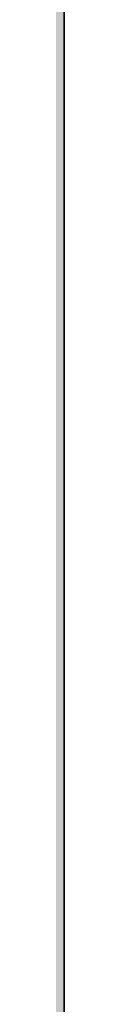
# Model space of a CAD drawing. Units: inches. Extents: x 2091 to 2899, y 967 to 2217.
# Tile 60 of 256: x 2212.1436 to 2212.1436, y 1099.9988 to 1100.1654. Entities that reach past the tile are written whole.
import ezdxf

# ---------------------------------------------------------------- set-up
doc = ezdxf.new("R2010")
doc.units = ezdxf.units.IN
doc.layers.add('A-WALL', color=7, linetype='Continuous', lineweight=35)
doc.layers.add('A-WALL-PATT', color=141, linetype='Continuous', lineweight=13, true_color=0xadddf7)

msp = doc.modelspace()

# ---------------------------------------------------------------- hatches: boundary and pattern name
at = {"layer": 'A-WALL-PATT'}
h = msp.add_hatch(color=256, dxfattribs=at)
h.dxf.hatch_style = 1
h.paths.add_polyline_path([(2212.1436, 1941.41906), (2387.6436, 1941.41906), (2387.6436, 1824.41906), (2392.1436, 1824.41906), (2392.1436, 1941.41906), (2609.6436, 1941.41906), (2609.6436, 1825.91906), (2614.1436, 1825.91906), (2614.1436, 1941.41906), (2794.1436, 1941.41906), (2794.1436, 1928.76217), (2803.1436, 1928.76217), (2803.1436, 2050.91906), (2203.1436, 2050.91906), (2203.1436, 1900.75786), (2212.1436, 1900.75786)])
h.paths.add_polyline_path([(2212.1436, 1945.91906), (2212.1436, 2041.91906), (2794.1436, 2041.91906), (2794.1436, 1945.91906), (2402.24824, 1945.91906), (2401.10243, 1945.77583), (2398.70243, 1945.77583)], flags=16)
h.paths.add_polyline_path([(2230.22986, 1948.06279), (2227.34986, 1949.50279), (2225.90986, 1951.90279), (2223.98986, 1952.86279), (2223.02986, 1955.26279), (2222.06986, 1959.58279), (2222.06986, 1963.42279), (2223.02986, 1965.66279), (2223.98986, 1965.34279), (2225.58591, 1963.86075), (2226.91153, 1964.95726), (2226.94886, 1965.93879), (2227.77832, 1966.95214), (2228.19992, 1968.8787), (2230.70986, 1964.86279), (2233.58986, 1966.30279), (2233.60731, 1966.33187), (2233.77266, 1964.9382), (2234.6338, 1963.67647), (2235.02986, 1963.90279), (2236.28203, 1965.57236), (2235.98986, 1962.94279), (2237.95451, 1957.54), (2238.38986, 1957.90279), (2239.21586, 1960.30579), (2238.65457, 1966.38496), (2238.69279, 1966.43807), (2238.84058, 1967.49971), (2238.78029, 1967.68749), (2238.88054, 1967.78676), (2238.66686, 1966.25179), (2239.21586, 1960.30579), (2238.38986, 1957.90279), (2236.94986, 1956.70279), (2234.54986, 1949.98279)], flags=0)
h.paths.add_polyline_path([(2278.01197, 1948.06279), (2276.49643, 1947.87335), (2275.84983, 1947.68861), (2274.65197, 1947.10279)], flags=0)
h.paths.add_polyline_path([(2269.85197, 1955.74279), (2268.27618, 1956.62933), (2270.8673, 1956.3484), (2269.37197, 1958.14279), (2268.71496, 1959.19233), (2270.56983, 1958.72861), (2268.58073, 1961.90609), (2270.81197, 1960.89188), (2270.81197, 1963.42279), (2271.39331, 1964.77926), (2270.29176, 1966.1562), (2271.77197, 1965.66279), (2272.14139, 1966.52476), (2273.92983, 1965.92861), (2275.63039, 1968.0543), (2276.33194, 1966.72186), (2276.52043, 1966.95214), (2276.94203, 1968.8787), (2277.73429, 1967.61108), (2278.13989, 1969.46452), (2279.65912, 1967.03374), (2280.41197, 1966.78279), (2280.9493, 1967.58879), (2281.60983, 1967.36861), (2282.13327, 1968.15376), (2282.34924, 1966.33344), (2282.34985, 1966.33259), (2283.40755, 1968.09542), (2283.71263, 1965.52402), (2284.32022, 1964.63379), (2284.51181, 1964.88924), (2284.23497, 1965.70479), (2284.50047, 1967.31896), (2284.90794, 1965.41742), (2285.39631, 1966.06858), (2285.43283, 1966.29061), (2285.47334, 1966.17128), (2286.35392, 1967.34539), (2286.22201, 1966.15817), (2287.66349, 1968.08015), (2287.71397, 1968.44279), (2288.4816, 1969.01668), (2288.57399, 1968.7289), (2288.91746, 1969.06904), (2288.60683, 1966.83761), (2288.92873, 1963.35131), (2288.93497, 1963.35679), (2288.92973, 1963.34042), (2289.01528, 1962.41387), (2290.11122, 1963.87513), (2290.13283, 1963.94261), (2290.21767, 1964.01706), (2290.11122, 1963.87513), (2289.15583, 1960.89161), (2288.59404, 1959.25723), (2288.57197, 1959.10279), (2289.53197, 1960.54279), (2290.01197, 1962.46279), (2290.19184, 1962.64266), (2289.76983, 1959.68861), (2286.88983, 1957.28861), (2284.48983, 1950.56861), (2283.31466, 1950.04631), (2283.29197, 1949.98279), (2280.29006, 1948.64861), (2281.12983, 1948.64861), (2282.56983, 1948.16861), (2283.20473, 1948.06279), (2278.97197, 1948.06279), (2276.09197, 1949.50279), (2274.65197, 1951.90279), (2272.73197, 1952.86279)], flags=0)
h.paths.add_polyline_path([(2271.15887, 1958.02177), (2272.96983, 1955.84861), (2272.00983, 1960.16861), (2272.00983, 1964.00861), (2272.62443, 1965.44266), (2274.32802, 1963.86075), (2275.65365, 1964.95726), (2275.63774, 1964.53909), (2277.41223, 1966.00689), (2277.03297, 1965.15679), (2276.82992, 1964.9756), (2276.76601, 1963.29501), (2277.44964, 1962.66022), (2279.45197, 1964.86279), (2282.33197, 1966.30279), (2283.52983, 1966.88861), (2283.29451, 1966.77095), (2283.91299, 1963.8847), (2284.89925, 1964.44827), (2284.73197, 1962.94279), (2286.69662, 1957.54), (2287.13197, 1957.90279), (2287.54191, 1959.09539), (2287.7794, 1958.44231), (2285.68274, 1956.6951), (2285.8765, 1959.79534), (2284.73197, 1962.94279), (2284.89925, 1964.44827), (2283.91299, 1963.8847), (2284.22383, 1962.43412), (2283.42436, 1963.60548), (2281.60983, 1962.56861), (2281.12983, 1960.16861), (2282.08983, 1956.32861), (2283.04983, 1952.96861), (2282.56983, 1950.56861), (2280.16983, 1948.64861), (2279.88332, 1948.79187), (2278.97197, 1948.06279), (2278.97197, 1949.02279), (2278.67231, 1949.39737), (2277.28983, 1950.08861), (2275.84983, 1952.48861), (2273.92983, 1953.44861), (2272.48983, 1954.88861), (2271.92165, 1954.88861), (2271.77197, 1955.26279)], flags=0)
h.paths.add_polyline_path([(2311.99415, 1955.74279), (2312.06272, 1955.67422), (2312.0551, 1955.7085)], flags=0)
h.paths.add_polyline_path([(2331.95615, 1963.95179), (2333.39615, 1965.39179), (2331.07715, 1963.35679), (2330.9986, 1963.11152)], flags=0)
h.paths.add_polyline_path([(2310.55415, 1954.30279), (2307.03981, 1956.27994), (2310.7629, 1955.87628), (2312.47415, 1953.82279), (2313.43415, 1951.42279), (2315.35415, 1950.46279), (2316.79415, 1948.06279), (2317.46615, 1947.72679), (2319.36869, 1947.96461), (2317.75415, 1949.98279), (2317.56953, 1950.61048), (2316.79415, 1951.90279), (2314.87415, 1952.86279), (2313.91415, 1955.26279), (2311.51415, 1958.14279), (2309.37549, 1961.55917), (2311.51415, 1960.33708), (2311.51415, 1961.98279), (2310.60467, 1963.11963), (2311.72661, 1962.47853), (2312.41833, 1964.09256), (2312.25596, 1964.29552), (2313.19415, 1963.98279), (2313.91415, 1965.66279), (2314.64678, 1965.41858), (2315.35415, 1966.30279), (2316.79415, 1967.74279), (2316.15744, 1966.9469), (2317.03411, 1965.28186), (2317.2226, 1965.51214), (2317.77705, 1968.04577), (2318.47411, 1966.72186), (2318.6626, 1966.95214), (2319.0842, 1968.8787), (2321.20705, 1965.48215), (2322.16142, 1966.9137), (2322.55415, 1966.78279), (2322.78599, 1967.13056), (2322.88165, 1966.32429), (2323.31204, 1965.72174), (2323.65129, 1965.89136), (2324.3965, 1967.13338), (2324.65694, 1964.9382), (2324.97199, 1964.47661), (2325.38728, 1967.0015), (2325.94081, 1964.41835), (2327.22893, 1966.13584), (2327.16632, 1965.57236), (2328.05914, 1966.76278), (2328.22458, 1966.24749), (2329.66797, 1967.67691), (2329.66458, 1967.68749), (2329.76482, 1967.78676), (2329.55115, 1966.25179), (2330.10015, 1960.30579), (2329.33281, 1958.07347), (2329.31306, 1957.93523), (2329.63415, 1958.20279), (2330.23415, 1959.10279), (2330.71415, 1961.02279), (2331.03415, 1961.34279), (2330.71415, 1959.10279), (2329.63415, 1958.20279), (2329.27415, 1957.66279), (2327.71211, 1956.3611), (2325.43415, 1949.98279), (2324.33377, 1949.49374), (2323.99415, 1948.54279), (2319.67415, 1946.62279), (2316.79415, 1948.06279), (2315.35415, 1950.46279), (2313.43415, 1951.42279)], flags=0)
h.paths.add_polyline_path([(2321.33568, 1947.95202), (2321.11415, 1948.06279), (2321.11415, 1949.02279), (2319.19415, 1951.42279), (2316.79415, 1959.58279), (2316.66324, 1959.58279), (2315.35415, 1958.14279), (2314.39415, 1958.14279), (2313.1483, 1958.70908), (2312.95415, 1959.58279), (2312.95415, 1960.89188), (2315.83415, 1959.58279), (2316.66324, 1959.58279), (2317.31471, 1960.29941), (2315.0302, 1962.42075), (2316.35582, 1963.51726), (2316.37234, 1963.95162), (2316.4702, 1963.86075), (2317.79582, 1964.95726), (2317.75522, 1963.88969), (2319.17515, 1965.15679), (2319.49841, 1965.88137), (2321.11415, 1965.34279), (2323.23589, 1962.37236), (2325.68635, 1963.77262), (2325.54279, 1962.48058), (2325.19878, 1963.49401), (2324.47851, 1963.08243), (2324.92601, 1960.99412), (2324.07809, 1962.23647), (2322.41479, 1961.28602), (2322.07415, 1959.58279), (2323.03415, 1955.74279), (2323.99415, 1952.38279), (2323.51415, 1949.98279), (2322.14272, 1948.88565), (2322.07415, 1948.54279)], flags=0)
h.paths.add_polyline_path([(2320.20748, 1963.33746), (2320.15415, 1963.42279), (2320.39415, 1963.54279)], flags=0)
h.paths.add_polyline_path([(2353.85053, 1965.8105), (2354.03053, 1965.7505), (2354.33053, 1966.4505), (2354.33053, 1966.9305)], flags=0)
h.paths.add_polyline_path([(2359.02058, 1969.02641), (2359.09838, 1968.90193), (2359.23353, 1969.5195), (2359.23353, 1969.9995)], flags=0)
h.paths.add_polyline_path([(2358.25669, 1966.68167), (2357.9836, 1966.34803), (2358.21127, 1966.14617), (2358.41049, 1966.38957)], flags=0)
h.paths.add_polyline_path([(2357.76847, 1966.05878), (2357.7322, 1965.10497), (2357.75105, 1965.12056), (2357.76953, 1965.6065), (2357.76953, 1966.05784)], flags=0)
h.paths.add_polyline_path([(2359.11153, 1965.3045), (2359.11153, 1964.8245), (2359.84453, 1966.4675), (2359.84453, 1966.9475)], flags=0)
h.paths.add_polyline_path([(2360.22368, 1966.62145), (2360.69853, 1969.3625), (2360.69853, 1969.8425), (2360.21053, 1967.0255), (2360.21053, 1966.6425)], flags=0)
h.paths.add_polyline_path([(2363.45053, 1967.8905), (2363.45053, 1968.3705), (2362.49053, 1966.9305), (2362.65604, 1966.69878)], flags=0)
h.paths.add_polyline_path([(2364.47552, 1966.07883), (2365.85053, 1968.3705), (2365.85053, 1968.8505), (2364.42798, 1966.47958)], flags=0)
h.paths.add_polyline_path([(2366.31353, 1965.8525), (2366.36671, 1965.69583), (2366.80253, 1968.3455), (2366.80253, 1968.8255)], flags=0)
h.paths.add_polyline_path([(2367.16531, 1965.80354), (2367.29053, 1966.9305), (2367.29053, 1967.4105), (2367.1027, 1965.72007)], flags=0)
h.paths.add_polyline_path([(2370.03653, 1959.9735), (2371.01353, 1963.0245), (2371.01353, 1963.5045), (2370.03653, 1960.4535)], flags=0)
h.paths.add_polyline_path([(2371.61053, 1960.2105), (2372.57053, 1961.6505), (2372.57053, 1962.1305), (2371.80253, 1960.9785)], flags=0)
h.paths.add_polyline_path([(2350.87367, 1956.00509), (2351.93053, 1955.8905), (2354.49053, 1953.3305), (2353.85053, 1954.9305), (2351.45053, 1957.8105), (2347.93553, 1963.4255), (2347.93553, 1963.9055), (2351.45053, 1958.2905), (2353.70507, 1955.58505), (2352.89053, 1959.2505), (2352.89053, 1959.7305), (2352.89053, 1961.92479), (2356.73053, 1959.7305), (2358.45447, 1961.62684), (2354.81053, 1965.0105), (2355.03086, 1965.28591), (2358.69109, 1961.88712), (2361.53053, 1965.0105), (2364.3765, 1966.43348), (2364.52439, 1965.18691), (2365.45447, 1963.82418), (2365.88107, 1964.06795), (2365.37053, 1966.4505), (2365.37053, 1966.9305), (2366.81053, 1960.2105), (2366.81053, 1959.7305), (2366.38871, 1952.98141), (2367.77053, 1956.8505), (2368.64123, 1957.57608), (2366.81053, 1962.6105), (2366.81053, 1963.0905), (2368.77518, 1957.68771), (2369.21053, 1958.0505), (2370.00159, 1960.35187), (2369.47523, 1966.05267), (2369.51346, 1966.10578), (2369.51417, 1966.11091), (2369.47523, 1966.53267), (2369.51346, 1966.58578), (2369.61463, 1967.31259), (2369.18253, 1968.6585), (2369.18253, 1969.1385), (2369.60096, 1967.83519), (2369.7012, 1967.93447), (2369.71795, 1968.05474), (2370.14518, 1968.37414), (2369.77871, 1968.01122), (2369.7012, 1967.45447), (2370.46816, 1968.214), (2369.67494, 1967.26577), (2369.51417, 1966.11091), (2370.03653, 1960.4535), (2370.03653, 1959.9735), (2369.44176, 1958.24319), (2370.65053, 1959.2505), (2371.04582, 1962.01756), (2371.13053, 1962.1305), (2370.65053, 1958.7705), (2367.77053, 1956.3705), (2365.37053, 1949.6505), (2362.0791, 1948.18764), (2363.45053, 1947.7305), (2361.05053, 1947.7305), (2360.09053, 1947.7305), (2357.10386, 1947.35717), (2360.09053, 1948.2105), (2358.17053, 1949.1705), (2356.73053, 1951.5705), (2354.81053, 1952.5305), (2351.93053, 1955.4105)], flags=0)
h.paths.add_polyline_path([(2361.05053, 1948.6905), (2359.13053, 1951.0905), (2356.73053, 1959.2505), (2355.77053, 1959.2505), (2352.89053, 1960.55959), (2352.89053, 1961.44479), (2355.89053, 1959.7305), (2356.73053, 1959.7305), (2356.83719, 1959.36783), (2361.53053, 1964.5305), (2363.24842, 1965.38945), (2364.92531, 1963.0418), (2362.49053, 1961.6505), (2362.06386, 1959.51717), (2362.97053, 1955.8905), (2363.93053, 1952.5305), (2363.93053, 1952.0505), (2363.45053, 1949.6505), (2361.05053, 1947.7305)], flags=0)
h.paths.add_polyline_path([(2359.13053, 1951.5705), (2359.29053, 1951.3705), (2361.05053, 1954.4505), (2361.05053, 1954.9305)], flags=0)
h.paths.add_polyline_path([(2357.21953, 1966.5455), (2356.79253, 1968.8145), (2356.79253, 1969.2945), (2357.21953, 1967.0255)], flags=0)
h.paths.add_polyline_path([(2361.05053, 1954.4505), (2361.53053, 1958.7705), (2361.53053, 1959.2505), (2361.05053, 1954.9305)], flags=0)
h.paths.add_polyline_path([(2402.54829, 1948.48608), (2402.30243, 1948.41583), (2402.59043, 1948.41583)], flags=0)
h.paths.add_polyline_path([(2394.14243, 1956.09583), (2395.68505, 1954.55321), (2396.7205, 1953.97068), (2396.06243, 1955.61583), (2395.24138, 1956.6011), (2395.8789, 1956.44171), (2395.10243, 1959.93583), (2395.10243, 1963.77583), (2396.06243, 1966.01583), (2397.02243, 1965.69583), (2398.61848, 1964.21379), (2399.94411, 1965.3103), (2399.98143, 1966.29183), (2400.81089, 1967.30518), (2401.23249, 1969.23174), (2403.53795, 1965.54301), (2403.94198, 1967.38932), (2404.70243, 1967.13583), (2405.46033, 1966.07478), (2406.62243, 1966.65583), (2406.63988, 1966.68491), (2406.80523, 1965.29124), (2406.92569, 1965.11475), (2407.34243, 1964.97583), (2407.87433, 1965.77367), (2408.1691, 1964.39805), (2409.31461, 1965.9254), (2409.21746, 1965.05105), (2409.44523, 1963.13124), (2410.30637, 1961.86951), (2410.70243, 1962.09583), (2411.44227, 1963.08228), (2411.16543, 1963.89783), (2411.61643, 1966.63976), (2411.72536, 1966.79111), (2411.87315, 1967.85275), (2411.81286, 1968.04053), (2411.91311, 1968.1398), (2411.69943, 1966.60483), (2412.24843, 1960.65883), (2413.22543, 1963.70983), (2414.3779, 1964.72116), (2414.51315, 1965.69275), (2414.45286, 1965.88053), (2414.55311, 1965.9798), (2414.3779, 1964.72116), (2414.51982, 1964.8457), (2414.36536, 1964.63111), (2414.33943, 1964.44483), (2414.88843, 1958.49883), (2414.06243, 1956.09583), (2412.62243, 1954.89583), (2410.17137, 1948.03285), (2410.01672, 1948.0844), (2405.90243, 1946.25583), (2405.90243, 1947.21583), (2405.20425, 1948.08856), (2404.22243, 1948.41583), (2403.26243, 1948.41583), (2400.38243, 1949.85583), (2399.66243, 1951.05583), (2397.98243, 1952.73583), (2397.02243, 1953.21583), (2395.68505, 1954.55321), (2392.65678, 1956.25691)], flags=0)
h.paths.add_polyline_path([(2409.08565, 1964.40744), (2409.13036, 1964.27572), (2409.26243, 1964.49583)], flags=0)
h.paths.add_polyline_path([(2397.74243, 1961.61583), (2398.70243, 1963.85583), (2399.66243, 1963.53583), (2401.42656, 1965.74099), (2401.79142, 1966.5588), (2402.07143, 1965.07083), (2402.83551, 1964.39337), (2403.2624, 1964.9149), (2403.33812, 1964.77109), (2402.61552, 1963.97622), (2402.49861, 1960.90224), (2403.543, 1959.93245), (2404.4132, 1960.88968), (2404.70243, 1962.33583), (2407.91635, 1964.17235), (2409.52021, 1961.92694), (2410.98708, 1957.89304), (2411.42243, 1958.25583), (2412.04796, 1960.07562), (2412.41034, 1959.07909), (2411.67562, 1958.46682), (2411.66243, 1958.25583), (2411.62607, 1958.42553), (2409.98243, 1957.05583), (2407.58243, 1950.33583), (2403.26243, 1948.41583), (2403.26243, 1949.37583), (2401.34243, 1951.77583), (2399.41651, 1958.32398), (2397.74243, 1959.08492), (2397.74243, 1959.97012), (2397.10243, 1960.33583), (2397.74243, 1960.04492)], flags=0)
h.paths.add_polyline_path([(2405.90243, 1952.97583), (2405.95043, 1953.40783), (2406.01672, 1953.17583)], flags=0)
h.paths.add_polyline_path([(2449.81778, 1967.11401), (2449.75232, 1967.13583), (2449.7937, 1967.0779)], flags=0)
h.paths.add_polyline_path([(2451.6977, 1966.61812), (2451.74089, 1966.69012), (2451.69205, 1966.6657)], flags=0)
h.paths.add_polyline_path([(2454.34363, 1965.73757), (2455.75232, 1967.61583), (2455.99232, 1968.09583), (2454.3645, 1965.9254)], flags=0)
h.paths.add_polyline_path([(2457.54732, 1968.86383), (2457.78732, 1969.34383), (2457.05432, 1968.79583), (2457.00762, 1968.46034)], flags=0)
h.paths.add_polyline_path([(2456.92178, 1967.85666), (2456.80224, 1968.22902), (2456.723, 1967.6598)], flags=0)
h.paths.add_polyline_path([(2457.30232, 1967.37683), (2457.54232, 1967.85683), (2456.81032, 1966.83983), (2456.74052, 1966.70022), (2456.74902, 1966.60811)], flags=0)
h.paths.add_polyline_path([(2458.27532, 1963.70983), (2458.15534, 1963.33515), (2460.35432, 1965.26483), (2460.59432, 1965.74483)], flags=0)
h.paths.add_polyline_path([(2458.39232, 1962.81583), (2458.36409, 1962.61819), (2459.59232, 1964.25583), (2459.83232, 1964.73583)], flags=0)
h.paths.add_polyline_path([(2459.35232, 1962.81583), (2459.27232, 1962.49583), (2460.07232, 1963.29583), (2460.31232, 1963.77583)], flags=0)
h.paths.add_polyline_path([(2458.68032, 1960.60783), (2458.63232, 1960.41583), (2459.59232, 1961.85583), (2459.83232, 1962.33583)], flags=0)
h.paths.add_polyline_path([(2437.83817, 1956.24265), (2439.19232, 1956.09583), (2441.35232, 1953.93583), (2440.87232, 1955.13583), (2438.47232, 1958.01583), (2438.07156, 1958.65602), (2438.71232, 1958.49583), (2440.6396, 1956.18311), (2439.91232, 1959.45583), (2439.91232, 1963.29583), (2441.35232, 1966.65583), (2441.59232, 1967.13583), (2441.11232, 1966.01583), (2442.07232, 1965.69583), (2443.98899, 1968.09167), (2444.24132, 1966.75083), (2444.9168, 1966.15192), (2445.67657, 1967.08014), (2446.25532, 1969.72483), (2446.49532, 1970.20483), (2446.28238, 1969.23174), (2447.36267, 1967.50327), (2447.72032, 1969.56783), (2447.96032, 1970.04783), (2447.48548, 1967.30678), (2448.79232, 1965.21583), (2448.47232, 1964.86383), (2448.55232, 1964.73583), (2451.45205, 1966.1857), (2451.61512, 1964.81124), (2452.30792, 1963.79617), (2453.23451, 1964.32565), (2454.07232, 1960.41583), (2453.62869, 1953.31765), (2454.79232, 1956.57583), (2455.03232, 1957.05583), (2455.71884, 1957.62793), (2453.83232, 1962.81583), (2453.94097, 1963.79362), (2453.33532, 1965.57783), (2453.82432, 1968.55083), (2454.06432, 1969.03083), (2453.57532, 1966.05783), (2454.04033, 1964.68792), (2453.83232, 1962.81583), (2455.71884, 1957.62793), (2456.36721, 1958.16824), (2457.05832, 1960.17883), (2457.29832, 1960.65883), (2456.47232, 1958.25583), (2457.71773, 1959.29367), (2457.67232, 1958.97583), (2454.88995, 1956.65719), (2453.61414, 1953.08492), (2453.59232, 1952.73583), (2453.35232, 1952.25583), (2453.3596, 1952.3722), (2452.63232, 1950.33583), (2452.39232, 1949.85583), (2449.20375, 1948.43869), (2450.71232, 1947.93583), (2448.07232, 1947.93583), (2447.11232, 1947.93583), (2444.55232, 1947.61583), (2447.1996, 1948.3722), (2445.19232, 1949.37583), (2443.75232, 1951.77583), (2441.83232, 1952.73583), (2438.95232, 1955.61583)], flags=0)
h.paths.add_polyline_path([(2443.99232, 1959.93583), (2444.04032, 1959.77263), (2444.12155, 1959.86199)], flags=0)
h.paths.add_polyline_path([(2442.91232, 1959.93583), (2443.03232, 1959.93583), (2442.44566, 1960.2025)], flags=0)
h.paths.add_polyline_path([(2444.98294, 1965.01968), (2445.27932, 1965.26483), (2445.51932, 1965.74483), (2444.994, 1965.3103)], flags=0)
h.paths.add_polyline_path([(2446.13332, 1965.02983), (2446.33037, 1965.4715), (2444.97032, 1964.25783), (2444.73032, 1963.77783)], flags=0)
h.paths.add_polyline_path([(2442.79232, 1959.45583), (2443.75232, 1959.45583), (2446.15232, 1951.29583), (2446.41232, 1951.75083), (2446.39232, 1951.77583), (2448.0806, 1954.73032), (2448.55232, 1958.97583), (2441.83232, 1965.21583), (2442.15495, 1965.61911), (2448.79232, 1959.45583), (2448.31232, 1955.13583), (2448.07232, 1954.65583), (2446.41232, 1951.75083), (2448.31232, 1949.37583), (2448.31232, 1948.41583), (2450.54089, 1950.19869), (2450.95232, 1952.25583), (2449.99232, 1955.61583), (2449.03232, 1959.45583), (2449.51232, 1961.85583), (2449.75232, 1962.33583), (2449.6749, 1961.94874), (2452.99451, 1963.84565), (2453.06441, 1963.51941), (2452.88461, 1963.78285), (2449.6749, 1961.94874), (2449.27232, 1959.93583), (2450.23232, 1956.09583), (2451.19232, 1952.73583), (2450.71232, 1950.33583), (2450.47232, 1949.85583), (2448.07232, 1947.93583), (2448.07232, 1948.53583), (2445.43232, 1949.85583), (2443.99232, 1952.25583), (2442.07232, 1953.21583), (2441.11232, 1955.61583), (2440.15232, 1959.93583), (2440.15232, 1960.65583)], flags=0)
h.paths.add_polyline_path([(2456.69232, 1966.98583), (2457.60832, 1968.08083), (2457.84832, 1968.56083), (2456.93232, 1967.46583)], flags=0)
h.paths.add_polyline_path([(2489.89657, 1966.58024), (2489.94295, 1966.18935), (2490.74749, 1967.53025), (2491.31912, 1968.95116)], flags=0)
h.paths.add_polyline_path([(2473.56247, 1956.40713), (2477.13998, 1956.01926), (2476.95533, 1956.24083), (2475.10805, 1957.28011), (2476.34749, 1956.97025), (2475.1869, 1958.82422), (2476.91912, 1958.39116), (2475.41164, 1960.79927), (2477.78749, 1959.71934), (2477.78749, 1962.25025), (2477.6374, 1962.43786), (2477.82255, 1962.33206), (2478.35912, 1963.58406), (2478.35912, 1963.67116), (2477.32435, 1964.96463), (2478.71483, 1964.50114), (2479.31912, 1965.91116), (2480.27912, 1965.59116), (2481.78397, 1967.47221), (2482.11649, 1965.70525), (2482.88056, 1965.02778), (2483.20931, 1965.42941), (2483.22017, 1965.71509), (2483.07594, 1965.98902), (2483.71176, 1966.76581), (2484.13049, 1968.67925), (2484.70212, 1970.10016), (2484.48918, 1969.12707), (2486.5029, 1965.90511), (2487.38749, 1965.61025), (2488.15342, 1966.75914), (2488.71702, 1965.97011), (2489.20009, 1966.21164), (2489.33067, 1965.11099), (2490.3939, 1963.62246), (2490.66077, 1963.77496), (2490.49391, 1964.55364), (2490.92306, 1963.92484), (2491.31912, 1964.15116), (2491.33339, 1964.17018), (2491.21049, 1964.53225), (2491.28176, 1964.96554), (2491.42579, 1964.29338), (2494.07648, 1967.82763), (2494.49792, 1966.51494), (2494.59817, 1966.61422), (2494.68949, 1967.27025), (2495.10675, 1967.5822), (2495.12984, 1967.74807), (2495.06955, 1967.93585), (2495.1698, 1968.03513), (2495.03178, 1967.04363), (2495.75382, 1967.75868), (2494.98205, 1966.68644), (2494.95612, 1966.50016), (2495.47902, 1960.83685), (2495.91049, 1962.18425), (2496.48212, 1963.60516), (2496.07269, 1962.32659), (2496.7689, 1962.93754), (2496.59912, 1962.71116), (2496.11912, 1959.35116), (2496.73287, 1960.27179), (2496.98749, 1961.29025), (2497.55912, 1962.71116), (2497.07912, 1960.79116), (2496.50749, 1959.37025), (2495.54749, 1957.93025), (2492.75884, 1955.60638), (2490.83912, 1950.23116), (2490.26749, 1948.81025), (2485.94749, 1946.89025), (2483.06749, 1948.33025), (2481.62749, 1950.73025), (2479.70749, 1951.69025), (2476.82749, 1954.57025)], flags=0)
h.paths.add_polyline_path([(2485.57697, 1948.31339), (2485.55912, 1948.31116), (2485.57876, 1948.31116)], flags=0)
h.paths.add_polyline_path([(2478.64506, 1954.55116), (2478.10904, 1956.96326), (2479.31912, 1955.51116), (2480.27912, 1953.11116), (2482.19912, 1952.15116), (2483.63912, 1949.75116), (2486.51912, 1948.31116), (2486.51912, 1949.27116), (2484.73931, 1951.49593), (2484.02749, 1950.25025), (2481.62749, 1958.41025), (2482.37515, 1959.23267), (2482.19912, 1959.83116), (2483.19757, 1960.92946), (2479.70749, 1964.17025), (2480.60336, 1965.29008), (2481.87517, 1964.10911), (2482.66639, 1964.76358), (2482.61536, 1963.4218), (2482.9892, 1963.07466), (2484.00849, 1963.98425), (2484.68361, 1965.49751), (2484.58012, 1965.40516), (2485.35727, 1967.14711), (2485.12065, 1965.7812), (2486.42749, 1963.69025), (2488.14538, 1964.5492), (2489.82227, 1962.20155), (2490.74749, 1962.73025), (2491.99966, 1964.39981), (2492.07605, 1965.08726), (2492.21289, 1964.68412), (2492.48537, 1965.04743), (2492.27912, 1963.19116), (2494.24377, 1957.78837), (2494.5625, 1958.05398), (2494.93349, 1959.13325), (2495.50512, 1960.55416), (2494.67912, 1958.15116), (2494.10749, 1956.73025), (2494.5625, 1958.05398), (2493.40854, 1957.09235), (2491.70749, 1961.77025), (2491.99966, 1964.39981), (2490.74749, 1962.73025), (2487.71203, 1960.9957), (2487.47912, 1959.83116), (2488.43912, 1955.99116), (2489.39912, 1952.63116), (2488.91912, 1950.23116), (2488.57692, 1949.9574), (2488.34749, 1948.81025), (2487.65172, 1948.25363), (2487.47912, 1948.31116), (2486.51912, 1948.31116), (2483.63912, 1949.75116), (2482.19912, 1952.15116), (2480.27912, 1953.11116), (2478.83912, 1954.55116)], flags=0)
h.paths.add_polyline_path([(2526.64825, 1966.98752), (2526.51734, 1967.03116), (2526.6001, 1966.9153)], flags=0)
h.paths.add_polyline_path([(2528.47064, 1966.44666), (2528.57449, 1966.61973), (2528.45707, 1966.56102)], flags=0)
h.paths.add_polyline_path([(2534.13334, 1967.49616), (2534.15669, 1967.54285), (2534.05984, 1967.4083)], flags=0)
h.paths.add_polyline_path([(2536.16192, 1964.0506), (2535.15734, 1962.71116), (2535.10087, 1962.31587), (2536.11734, 1963.67116), (2536.42053, 1964.27754)], flags=0)
h.paths.add_polyline_path([(2535.15734, 1959.83116), (2536.11734, 1961.27116), (2536.59734, 1962.23116), (2535.25334, 1960.21516)], flags=0)
h.paths.add_polyline_path([(2513.24904, 1956.2848), (2516.22118, 1955.96256), (2514.99734, 1957.43116), (2514.19582, 1958.71154), (2515.47734, 1958.39116), (2516.93189, 1956.64571), (2516.43734, 1958.87116), (2516.43734, 1962.71116), (2516.87269, 1963.72697), (2515.34643, 1965.6348), (2517.39734, 1964.95116), (2517.87734, 1966.07116), (2518.35734, 1967.03116), (2517.87734, 1965.91116), (2518.83734, 1965.59116), (2520.48659, 1967.65272), (2520.76634, 1966.16616), (2521.53042, 1965.48869), (2521.78144, 1965.79537), (2521.80091, 1966.30727), (2521.4778, 1966.92094), (2521.24634, 1967.12616), (2521.1777, 1967.49091), (2521.4778, 1966.92094), (2522.01042, 1966.44869), (2522.25739, 1966.75042), (2522.78034, 1969.14016), (2523.26034, 1970.10016), (2523.0474, 1969.12707), (2524.67313, 1966.5259), (2526.03734, 1966.07116), (2526.79524, 1965.01011), (2527.97707, 1965.60102), (2528.14014, 1964.22657), (2528.66459, 1963.45816), (2529.38862, 1963.87189), (2529.32967, 1964.14699), (2529.48128, 1963.92484), (2529.87734, 1964.15116), (2529.98401, 1964.29338), (2529.78905, 1965.20318), (2530.0624, 1964.3979), (2532.80248, 1968.05135), (2533.14777, 1966.97585), (2533.24802, 1967.07513), (2533.33934, 1967.73116), (2533.67285, 1967.98049), (2533.72802, 1968.03513), (2533.51434, 1966.50016), (2534.02472, 1960.9725), (2534.56034, 1962.64516), (2535.04034, 1963.60516), (2534.06334, 1960.55416), (2533.23734, 1958.15116), (2534.28815, 1959.02684), (2534.19734, 1958.39116), (2531.5126, 1956.15387), (2529.39734, 1950.23116), (2528.91734, 1949.27116), (2526.44877, 1948.17402), (2527.47734, 1947.83116), (2530.35734, 1947.35116), (2524.59734, 1947.35116), (2521.71734, 1948.79116), (2520.27734, 1951.19116), (2518.35734, 1952.15116), (2515.47734, 1955.03116)], flags=0)
h.paths.add_polyline_path([(2523.93476, 1967.19031), (2523.61951, 1966.48369), (2523.7705, 1966.24211)], flags=0)
h.paths.add_polyline_path([(2518.83734, 1953.11116), (2517.87734, 1955.51116), (2516.88498, 1959.97678), (2516.91734, 1959.96207), (2516.91734, 1962.02545), (2520.75734, 1959.83116), (2522.02495, 1961.22553), (2518.35734, 1964.63116), (2519.00259, 1965.43772), (2520.43339, 1964.10911), (2521.30112, 1964.82687), (2521.24516, 1963.35533), (2525.63831, 1959.27598), (2526.03734, 1961.27116), (2529.39734, 1963.19116), (2530.64952, 1964.86073), (2530.66472, 1964.99755), (2530.69196, 1964.91731), (2531.08778, 1965.44507), (2530.94599, 1964.16894), (2530.69196, 1964.91731), (2529.39734, 1963.19116), (2526.3625, 1961.45697), (2526.03734, 1959.83116), (2526.99734, 1955.99116), (2527.95734, 1952.63116), (2527.47734, 1950.23116), (2527.13449, 1949.95687), (2526.97393, 1949.15409), (2526.69734, 1949.03116), (2524.59734, 1947.35116), (2524.59734, 1948.31116), (2524.27734, 1948.71116), (2522.19734, 1949.75116), (2520.75734, 1952.15116)], flags=0)
h.paths.add_polyline_path([(2520.27734, 1958.87116), (2520.85334, 1959.50476), (2523.15734, 1951.67116), (2524.61389, 1954.22013), (2524.59734, 1954.07116), (2522.67734, 1950.71116)], flags=0)
h.paths.add_polyline_path([(2559.37091, 1966.31116), (2559.39841, 1966.32491), (2559.40194, 1966.3453)], flags=0)
h.paths.add_polyline_path([(2549.77091, 1957.19116), (2552.65091, 1954.31116), (2552.13399, 1955.60347), (2550.61091, 1957.43116), (2547.09591, 1963.04616), (2545.77591, 1965.20616), (2549.29091, 1959.59116), (2551.69091, 1956.71116), (2550.79293, 1960.75206), (2550.73091, 1960.78025), (2550.73091, 1964.87116), (2551.69091, 1967.11116), (2552.65091, 1966.79116), (2554.24696, 1965.30911), (2555.03425, 1965.96034), (2555.58167, 1966.64461), (2555.60991, 1967.38716), (2556.43937, 1968.40051), (2556.86097, 1970.32707), (2559.37091, 1966.31116), (2560.69091, 1964.15116), (2562.40881, 1965.01011), (2561.65091, 1966.07116), (2560.33091, 1968.23116), (2561.7585, 1966.23254), (2562.34721, 1967.11561), (2562.43371, 1966.38657), (2563.1278, 1965.3696), (2563.57091, 1965.59116), (2563.58836, 1965.62024), (2563.36254, 1967.52354), (2563.72249, 1965.84379), (2565.06, 1968.07298), (2564.73286, 1965.12872), (2565.11758, 1963.33338), (2567.44462, 1966.43611), (2567.31561, 1967.83333), (2567.35384, 1967.88644), (2567.50163, 1968.94807), (2567.44134, 1969.13585), (2567.54159, 1969.23513), (2567.32791, 1967.70016), (2567.87691, 1961.75416), (2568.74669, 1964.47033), (2568.63561, 1965.67333), (2568.67384, 1965.72644), (2568.82163, 1966.78807), (2568.76134, 1966.97585), (2568.86159, 1967.07513), (2568.64791, 1965.54016), (2568.72613, 1964.69303), (2568.85391, 1964.80516), (2568.74669, 1964.47033), (2568.81724, 1963.70626), (2568.97091, 1963.91116), (2568.86607, 1963.17731), (2569.19691, 1959.59416), (2568.37091, 1957.19116), (2566.93091, 1955.99116), (2564.62027, 1949.52137), (2564.65091, 1949.51116), (2564.61662, 1949.51116), (2564.53091, 1949.27116), (2560.21091, 1947.35116), (2557.33091, 1948.79116), (2556.0452, 1950.93402), (2556.01091, 1950.95116), (2555.85662, 1951.2083), (2553.97091, 1952.15116), (2551.09091, 1955.03116), (2546.65014, 1957.52951)], flags=0)
h.paths.add_polyline_path([(2567.02579, 1959.33023), (2567.03501, 1959.30489), (2567.05091, 1959.35116)], flags=0)
h.paths.add_polyline_path([(2551.96829, 1962.51837), (2553.01091, 1964.95116), (2553.97091, 1964.63116), (2555.56696, 1963.14911), (2556.89258, 1964.24563), (2556.92991, 1965.22716), (2557.14398, 1965.48869), (2556.42007, 1966.13056), (2556.39142, 1966.10499), (2556.37991, 1966.16616), (2556.42007, 1966.13056), (2556.95191, 1966.60516), (2557.09214, 1966.91948), (2557.57087, 1966.01023), (2557.75937, 1966.24051), (2557.41791, 1964.68016), (2556.89258, 1964.24563), (2556.80709, 1961.99757), (2560.69091, 1958.39116), (2560.63553, 1957.8927), (2560.81091, 1957.19116), (2561.77091, 1953.83116), (2561.29091, 1951.43116), (2559.11042, 1949.68677), (2559.15648, 1949.62919), (2563.02652, 1951.34921), (2562.61091, 1949.27116), (2560.21091, 1947.35116), (2560.21091, 1948.31116), (2559.25091, 1949.51116), (2558.89091, 1949.51116), (2558.89091, 1949.96116), (2558.29091, 1950.71116), (2558.0537, 1951.51767), (2556.97091, 1952.87116), (2555.06788, 1959.34146), (2552.05091, 1961.06545), (2552.05091, 1962.47116)], flags=0)
h.paths.add_polyline_path([(2588.33005, 1958.39116), (2588.61025, 1958.11096), (2588.55336, 1958.36695)], flags=0)
h.paths.add_polyline_path([(2594.74545, 1950.49309), (2593.95753, 1953.17202), (2593.13005, 1954.55116), (2591.21005, 1955.51116), (2590.25005, 1957.91116), (2588.30903, 1960.24038), (2586.17731, 1961.20935), (2587.85005, 1960.79116), (2587.25342, 1961.74425), (2588.44131, 1961.06545), (2588.44131, 1962.65553), (2588.42168, 1962.66535), (2588.44131, 1962.71116), (2586.91404, 1964.62026), (2588.87709, 1963.72796), (2589.29005, 1964.69154), (2589.29005, 1966.07116), (2590.25005, 1968.31116), (2591.21005, 1967.99116), (2592.8061, 1966.50911), (2594.13172, 1967.60563), (2594.16905, 1968.58716), (2594.99851, 1969.60051), (2595.4201, 1971.52707), (2597.93005, 1967.51116), (2600.81005, 1968.95116), (2600.8275, 1968.98024), (2600.99285, 1967.58657), (2601.85399, 1966.32484), (2602.10714, 1966.4695), (2602.23635, 1967.25507), (2602.35672, 1966.69338), (2603.50222, 1968.22073), (2603.21005, 1965.59116), (2605.1747, 1960.18837), (2605.50689, 1960.4652), (2605.02602, 1965.67333), (2605.06425, 1965.72644), (2605.21203, 1966.78807), (2605.15174, 1966.97585), (2605.25199, 1967.07513), (2605.34331, 1967.73116), (2605.9529, 1968.1869), (2605.87475, 1969.03333), (2605.91298, 1969.08644), (2606.06077, 1970.14807), (2606.00048, 1970.33585), (2606.10073, 1970.43513), (2605.88705, 1968.90016), (2606.43605, 1962.95416), (2605.61005, 1960.55116), (2605.99704, 1960.87365), (2606.56431, 1962.64516), (2608.24149, 1964.11694), (2608.01005, 1963.19116), (2607.05005, 1961.75116), (2606.63149, 1961.40236), (2606.20131, 1958.39116), (2603.32131, 1955.99116), (2600.92131, 1949.27116), (2596.60131, 1947.35116), (2593.72131, 1948.79116), (2592.85731, 1950.23116), (2592.65005, 1950.23116)], flags=0)
h.paths.add_polyline_path([(2596.60131, 1947.35116), (2596.60131, 1948.31116), (2594.68131, 1950.71116), (2596.15495, 1953.29003), (2595.53005, 1954.07116), (2593.19923, 1961.99596), (2592.65134, 1962.50471), (2591.78015, 1963.00253), (2593.28299, 1964.24563), (2593.32031, 1965.22716), (2594.14977, 1966.24051), (2594.57137, 1968.16707), (2596.18265, 1965.58902), (2596.95127, 1966.43451), (2598.04131, 1966.07116), (2598.79921, 1965.01011), (2599.96131, 1965.59116), (2599.97876, 1965.62024), (2600.14411, 1964.22657), (2601.00526, 1962.96484), (2601.40131, 1963.19116), (2602.65349, 1964.86073), (2602.36131, 1962.23116), (2603.79275, 1958.29472), (2601.97764, 1953.21243), (2601.94621, 1952.70945), (2599.46876, 1951.60836), (2599.00131, 1949.27116)], flags=0)
h.paths.add_polyline_path([(2597.56131, 1958.87116), (2597.67097, 1959.41942), (2597.59505, 1958.7362)], flags=0)
h.paths.add_polyline_path([(2623.6663, 1961.25438), (2625.51916, 1960.79116), (2624.96554, 1961.67553), (2627.19916, 1960.66025), (2627.19916, 1961.15116), (2626.95916, 1962.23116), (2626.95916, 1963.49116), (2625.58232, 1965.21221), (2626.95916, 1964.42545), (2626.95916, 1965.83116), (2626.86916, 1965.86116), (2627.91916, 1968.31116), (2628.87916, 1967.99116), (2630.47521, 1966.50911), (2631.80084, 1967.60563), (2631.83816, 1968.58716), (2632.66762, 1969.60051), (2633.08922, 1971.52707), (2635.59916, 1967.51116), (2638.47916, 1968.95116), (2638.49661, 1968.98024), (2638.66196, 1967.58657), (2639.17627, 1966.83301), (2639.78022, 1967.83958), (2640.02583, 1966.69338), (2641.17134, 1968.22073), (2640.87916, 1965.59116), (2641.11426, 1964.94463), (2641.41134, 1965.34073), (2641.3081, 1964.41159), (2642.84381, 1960.18837), (2643.27916, 1960.55116), (2644.08474, 1962.89474), (2643.78387, 1966.15333), (2643.80683, 1966.18524), (2643.60068, 1968.41805), (2643.52281, 1968.66058), (2643.72988, 1970.14807), (2643.66959, 1970.33585), (2643.76984, 1970.43513), (2643.55616, 1968.90016), (2643.60068, 1968.41805), (2643.90959, 1967.45585), (2644.00984, 1967.55513), (2643.81174, 1966.13208), (2644.10516, 1962.95416), (2644.23877, 1961.35084), (2644.71916, 1961.75116), (2645.03285, 1962.2217), (2645.32216, 1963.12516), (2646.07642, 1963.78705), (2645.03285, 1962.2217), (2644.34516, 1960.07416), (2643.51916, 1957.67116), (2642.07916, 1956.47116), (2639.71961, 1949.86442), (2639.87553, 1949.83843), (2635.35916, 1947.83116), (2632.47916, 1949.27116), (2631.03916, 1951.67116), (2629.11916, 1952.63116), (2628.15916, 1955.03116), (2625.75916, 1957.91116)], flags=0)
h.paths.add_polyline_path([(2627.81631, 1956.57402), (2627.37371, 1958.56571), (2626.37631, 1959.76259), (2627.19916, 1959.35116), (2627.37371, 1958.56571), (2627.91916, 1957.91116), (2628.87916, 1955.51116), (2630.79916, 1954.55116), (2632.23916, 1952.15116), (2633.31502, 1951.61323), (2631.03916, 1959.35116), (2631.49783, 1959.85569), (2630.79916, 1962.23116), (2631.44987, 1962.94694), (2630.71521, 1963.62911), (2632.04084, 1964.72563), (2632.07816, 1965.70716), (2632.29224, 1965.96869), (2631.70534, 1966.48907), (2633.13644, 1967.76614), (2633.32922, 1968.64707), (2634.67472, 1966.49427), (2635.20847, 1967.08139), (2636.79916, 1966.55116), (2637.6764, 1967.86702), (2638.99395, 1966.02246), (2639.70534, 1966.42898), (2641.11916, 1959.83116), (2640.93007, 1956.80571), (2639.43916, 1952.63116), (2638.22746, 1952.09262), (2637.75916, 1949.75116), (2635.35916, 1947.83116), (2635.35916, 1948.79116), (2633.43916, 1951.19116), (2633.31502, 1951.61323), (2632.23916, 1952.15116), (2630.79916, 1954.55116), (2628.87916, 1955.51116)], flags=0)
h.paths.add_polyline_path([(2637.75916, 1953.83116), (2637.27916, 1955.51116), (2636.31916, 1959.35116), (2636.79916, 1961.75116), (2639.23395, 1963.14246), (2637.55706, 1965.49011), (2638.73889, 1966.08102), (2638.90196, 1964.70657), (2639.7631, 1963.44484), (2636.79916, 1961.75116), (2636.5325, 1960.41783), (2637.03916, 1958.39116), (2637.99916, 1955.03116)], flags=0)
h.paths.add_polyline_path([(2668.56741, 1951.43116), (2667.60741, 1953.83116), (2665.20741, 1956.71116), (2662.2939, 1961.36531), (2665.44741, 1959.59116), (2666.64741, 1958.39116), (2666.64741, 1959.97516), (2666.05832, 1960.68207), (2666.64741, 1960.34545), (2666.64741, 1961.99116), (2666.70009, 1962.11409), (2666.40741, 1963.43116), (2666.40741, 1967.27116), (2667.36741, 1969.51116), (2668.32741, 1969.19116), (2669.92346, 1967.70911), (2671.24908, 1968.80563), (2671.28641, 1969.78716), (2672.11587, 1970.80051), (2672.53746, 1972.72707), (2675.04741, 1968.71116), (2677.92741, 1970.15116), (2677.94486, 1970.18024), (2678.11021, 1968.78657), (2678.97135, 1967.52484), (2679.36741, 1967.75116), (2680.61958, 1969.42073), (2680.32741, 1966.79116), (2682.29206, 1961.38837), (2682.72741, 1961.75116), (2683.35831, 1963.58657), (2683.23211, 1964.95333), (2683.27034, 1965.00644), (2683.39322, 1965.88914), (2683.35997, 1966.24921), (2683.35784, 1966.25585), (2683.35923, 1966.25723), (2682.99211, 1970.23333), (2683.03034, 1970.28644), (2683.17812, 1971.34807), (2683.11784, 1971.53585), (2683.21808, 1971.63513), (2683.00441, 1970.10016), (2683.35923, 1966.25723), (2683.45808, 1966.35513), (2683.39322, 1965.88914), (2683.41391, 1965.66502), (2684.42381, 1966.87227), (2683.55341, 1964.15416), (2683.35831, 1963.58657), (2683.79341, 1958.87416), (2682.96741, 1956.47116), (2681.52741, 1955.27116), (2680.10923, 1951.30025), (2680.08493, 1950.91157), (2679.97685, 1950.92959), (2679.12741, 1948.55116), (2674.80741, 1946.63116), (2671.92741, 1948.07116), (2670.48741, 1950.47116)], flags=0)
h.paths.add_polyline_path([(2671.93568, 1953.22702), (2671.68741, 1953.35116), (2670.24741, 1955.75116), (2668.32741, 1956.71116), (2667.35674, 1959.13783), (2669.52741, 1958.15116), (2670.48741, 1958.15116), (2671.47941, 1959.24236), (2670.6844, 1961.94538), (2668.8896, 1963.61198), (2667.30741, 1964.33116), (2668.56741, 1963.91116), (2668.83094, 1964.24057), (2670.24741, 1963.43116), (2672.42214, 1965.82337), (2672.77746, 1967.44707), (2673.23407, 1966.71649), (2674.41192, 1968.01212), (2673.98056, 1965.52211), (2675.28741, 1963.43116), (2675.55407, 1963.56449), (2675.93241, 1965.45616), (2676.24741, 1965.35116), (2677.0053, 1964.29011), (2678.16741, 1964.87116), (2679.60741, 1967.27116), (2680.32741, 1963.91116), (2680.30655, 1963.57748), (2680.34724, 1963.45761), (2680.85958, 1964.14073), (2680.56741, 1961.51116), (2681.10362, 1960.03657), (2678.88741, 1953.83116), (2677.09248, 1953.03341), (2677.68741, 1950.95116), (2677.20741, 1948.55116), (2674.80741, 1946.63116), (2674.80741, 1947.59116), (2672.88741, 1949.99116)], flags=0)
h.paths.add_polyline_path([(2673.98455, 1951.91116), (2674.56741, 1952.93116), (2674.56741, 1951.91116), (2676.96741, 1953.83116), (2677.44741, 1956.23116), (2676.48741, 1959.59116), (2676.24741, 1960.55116), (2679.72959, 1962.54098), (2680.05927, 1961.00248), (2679.21135, 1962.24484), (2676.24741, 1960.55116), (2676.48741, 1959.59116), (2677.44741, 1956.23116), (2676.96741, 1953.83116), (2674.56741, 1951.91116)], flags=0)
h.paths.add_polyline_path([(2707.47928, 1952.81465), (2706.51928, 1955.21465), (2705.55928, 1959.53465), (2705.55928, 1963.37465), (2706.51928, 1965.61465), (2707.47928, 1965.29465), (2709.07533, 1963.81261), (2710.40096, 1964.90912), (2710.43828, 1965.89065), (2711.26774, 1966.904), (2711.68934, 1968.83056), (2714.19928, 1964.81465), (2717.07928, 1966.25465), (2717.09673, 1966.28373), (2717.26208, 1964.89006), (2718.12322, 1963.62833), (2718.51928, 1963.85465), (2719.77146, 1965.52422), (2719.47928, 1962.89465), (2721.44393, 1957.49186), (2721.87928, 1957.85465), (2722.70528, 1960.25765), (2722.14399, 1966.33682), (2722.18221, 1966.38993), (2722.33, 1967.45157), (2722.26971, 1967.63934), (2722.36996, 1967.73862), (2722.15628, 1966.20365), (2722.70528, 1960.25765), (2721.87928, 1957.85465), (2720.43928, 1956.65465), (2718.03928, 1949.93465), (2713.71928, 1948.01465), (2710.83928, 1949.45465), (2709.39928, 1951.85465)], flags=0)
h.paths.add_polyline_path([(2749.30123, 1952.81465), (2748.34123, 1955.21465), (2747.38123, 1959.53465), (2747.38123, 1963.37465), (2748.34123, 1965.61465), (2749.30123, 1965.29465), (2750.89728, 1963.81261), (2752.2229, 1964.90912), (2752.26023, 1965.89065), (2753.08969, 1966.904), (2753.51129, 1968.83056), (2756.02123, 1964.81465), (2758.90123, 1966.25465), (2758.91868, 1966.28373), (2759.08403, 1964.89006), (2759.94517, 1963.62833), (2760.34123, 1963.85465), (2761.5934, 1965.52422), (2761.30123, 1962.89465), (2763.26588, 1957.49186), (2763.70123, 1957.85465), (2764.52723, 1960.25765), (2763.96594, 1966.33682), (2764.00416, 1966.38993), (2764.15195, 1967.45157), (2764.09166, 1967.63934), (2764.19191, 1967.73862), (2763.97823, 1966.20365), (2764.52723, 1960.25765), (2763.70123, 1957.85465), (2762.26123, 1956.65465), (2759.86123, 1949.93465), (2755.54123, 1948.01465), (2752.66123, 1949.45465), (2751.22123, 1951.85465)], flags=0)
h.paths.add_polyline_path([(2212.1436, 1819.93451), (2203.1436, 1819.93451), (2203.1436, 1739.97955), (2212.1436, 1739.97955), (2212.1436, 1780.91906), (2392.1436, 1780.91906), (2392.1436, 1783.91906), (2212.1436, 1783.91906)])
h.paths.add_polyline_path([(2803.1436, 1847.93882), (2794.1436, 1847.93882), (2794.1436, 1785.41906), (2609.6436, 1785.41906), (2493.87561, 1785.41906), (2493.87561, 1780.91906), (2609.6436, 1780.91906), (2794.1436, 1780.91906), (2794.1436, 1696.91906), (2609.37561, 1696.91906), (2609.37561, 1742.91906), (2604.87561, 1742.91906), (2604.87561, 1644.41906), (2609.37561, 1644.41906), (2609.37561, 1692.41906), (2794.1436, 1692.41906), (2794.1436, 1668.16474), (2803.1436, 1668.16474)])
h.paths.add_polyline_path([(2392.1436, 1740.41906), (2387.6436, 1740.41906), (2387.6436, 1629.41906), (2212.1436, 1629.41906), (2212.1436, 1659.1562), (2203.1436, 1659.1562), (2203.1436, 1494.08944), (2212.1436, 1494.08944), (2212.1436, 1627.91906), (2392.1436, 1627.91906)])
h.paths.add_polyline_path([(2457.87561, 1780.91906), (2453.37561, 1780.91906), (2453.37561, 1644.41906), (2568.87561, 1644.41906), (2568.87561, 1648.91906), (2457.87561, 1648.91906)])
h.paths.add_polyline_path([(2545.1436, 1591.91906), (2540.6436, 1591.91906), (2540.6436, 1567.91906), (2468.6436, 1567.91906), (2468.6436, 1627.91906), (2509.1436, 1627.91906), (2509.1436, 1632.41906), (2464.1436, 1632.41906), (2464.1436, 1563.41906), (2545.1436, 1563.41906)])
h.paths.add_polyline_path([(2268.6436, 1555.91906), (2212.1436, 1555.91906), (2212.1436, 1551.41906), (2268.6436, 1551.41906)], flags=17)
h.paths.add_polyline_path([(2212.1436, 1413.26609), (2203.1436, 1413.26609), (2203.1436, 1233.0704), (2212.1436, 1233.0704)])
h.paths.add_polyline_path([(2267.6436, 1351.91906), (2212.1436, 1351.91906), (2212.1436, 1347.41906), (2267.6436, 1347.41906)], flags=17)
h.paths.add_polyline_path([(2456.6436, 1489.41906), (2452.1436, 1489.41906), (2452.1436, 1351.91906), (2312.6436, 1351.91906), (2312.6436, 1347.41906), (2456.6436, 1347.41906)])
h.paths.add_polyline_path([(2472.37017, 1455.41906), (2467.87017, 1455.41906), (2467.87017, 1347.41906), (2472.37017, 1347.41906)])
h.paths.add_polyline_path([(2794.1436, 1351.91906), (2543.37017, 1351.91906), (2543.37017, 1347.41906), (2794.1436, 1347.41906)], flags=17)
h.paths.add_polyline_path([(2312.6436, 1347.41906), (2308.1436, 1347.41906), (2308.1436, 1302.16179), (2308.34197, 1302.16433), (2308.1436, 1298.16925), (2308.1436, 1275.41906), (2212.1436, 1275.41906), (2212.1436, 1270.91906), (2312.6436, 1270.91906)], flags=17)
h.paths.add_polyline_path([(2212.1436, 1152.24706), (2203.1436, 1152.24706), (2203.1436, 1090.91906), (2803.1436, 1090.91906), (2803.1436, 1392.71355), (2794.1436, 1392.71355), (2794.1436, 1143.41906), (2548.03245, 1143.41906), (2548.03245, 1138.91906), (2794.1436, 1138.91906), (2794.1436, 1099.91906), (2212.1436, 1099.91906)])
h.paths.add_polyline_path([(2471.53245, 1266.32853, 0.031658), (2467.03245, 1269.94579), (2467.03245, 1143.41906), (2471.53245, 1143.41906), (2471.53245, 1148.81906)], flags=17)
h.paths.add_polyline_path([(2803.1436, 1587.34139), (2794.1436, 1587.34139), (2794.1436, 1473.5369), (2803.1436, 1473.5369)])
h.paths.add_polyline_path([(2794.1436, 1536.41906), (2651.1436, 1536.41906), (2651.1436, 1531.91906), (2794.1436, 1531.91906)])
h.paths.add_polyline_path([(2614.1436, 1620.41906), (2609.6436, 1620.41906), (2609.6436, 1536.41906), (2614.1436, 1536.41906)])
h.paths.add_polyline_path([(2271.08273, 1964.31724), (2776.85297, 1964.31724), (2776.85297, 2037.16962), (2271.08273, 2037.16962)], flags=8)
h.paths.add_polyline_path([(2380.64929, 1536.82414), (2461.04081, 1536.82414), (2461.04081, 1554.65259), (2380.64929, 1554.65259)], flags=9)
h.paths.add_polyline_path([(2203.65504, 1608.81531), (2316.11844, 1608.81531), (2316.11844, 1621.91836), (2203.65504, 1621.91836)], flags=24)
h.paths.add_polyline_path([(2212.67726, 1313.5041), (2282.59152, 1313.5041), (2282.59152, 1322.74524), (2212.67726, 1322.74524)], flags=24)
h.paths.add_polyline_path([(2457.11198, 1114.77857), (2558.48158, 1114.77857), (2558.48158, 1142.21968), (2457.11198, 1142.21968)], flags=25)
h.paths.add_polyline_path([(2473.44234, 1273.01007), (2604.64123, 1273.01007), (2604.64123, 1318.34693), (2473.44234, 1318.34693)], flags=25)
h.paths.add_polyline_path([(2638.8763, 1626.97743), (2684.25037, 1627.97674), (2684.03848, 1637.59749), (2638.66442, 1636.59819)], flags=9)
h.paths.add_polyline_path([(2537.59055, 1453.79345), (2628.38955, 1453.79345), (2628.38955, 1475.34481), (2537.59055, 1475.34481)], flags=9)
h.paths.add_polyline_path([(2504.13764, 1714.6324), (2554.64719, 1714.6324), (2554.64719, 1730.23771), (2504.13764, 1730.23771)], flags=25)
h.paths.add_polyline_path([(2487.50118, 1575.65187), (2535.09712, 1575.65187), (2535.09712, 1598.37765), (2487.50118, 1598.37765)], flags=25)
h.paths.add_polyline_path([(2709.0994, 1735.71028), (2740.0166, 1735.71028), (2740.0166, 1749.93764), (2709.0994, 1749.93764)], flags=25)
h.paths.add_polyline_path([(2442.43842, 1792.17166), (2564.72884, 1792.17166), (2564.72884, 1842.00016), (2442.43842, 1842.00016)], flags=9)
h.paths.add_polyline_path([(2655.8158, 1809.64408), (2789.52014, 1806.6938), (2790.08498, 1832.29164), (2656.38064, 1835.24192)], flags=25)
h.paths.add_polyline_path([(2234.8427, 1797.72014), (2368.59285, 1794.76885), (2369.16072, 1820.50413), (2235.41056, 1823.45542)], flags=9)
h.paths.add_polyline_path([(2245.13847, 1644.00633), (2398.42773, 1640.6239), (2398.99484, 1666.32482), (2245.70557, 1669.70725)], flags=9)
h.paths.add_polyline_path([(2306.14285, 1431.16852), (2413.76831, 1428.79369), (2414.33315, 1454.39153), (2306.70768, 1456.76636)], flags=9)
h.paths.add_polyline_path([(2306.83458, 1458.23314), (2393.38048, 1456.32345), (2393.93281, 1481.35436), (2307.38691, 1483.26405)], flags=9)

# ---------------------------------------------------------------- linework, layer by layer
at = {"layer": 'A-WALL'}
msp.add_line((2212.1436, 1099.91906), (2212.1436, 1627.91906), dxfattribs=at)

doc.saveas('drawing.dxf')
